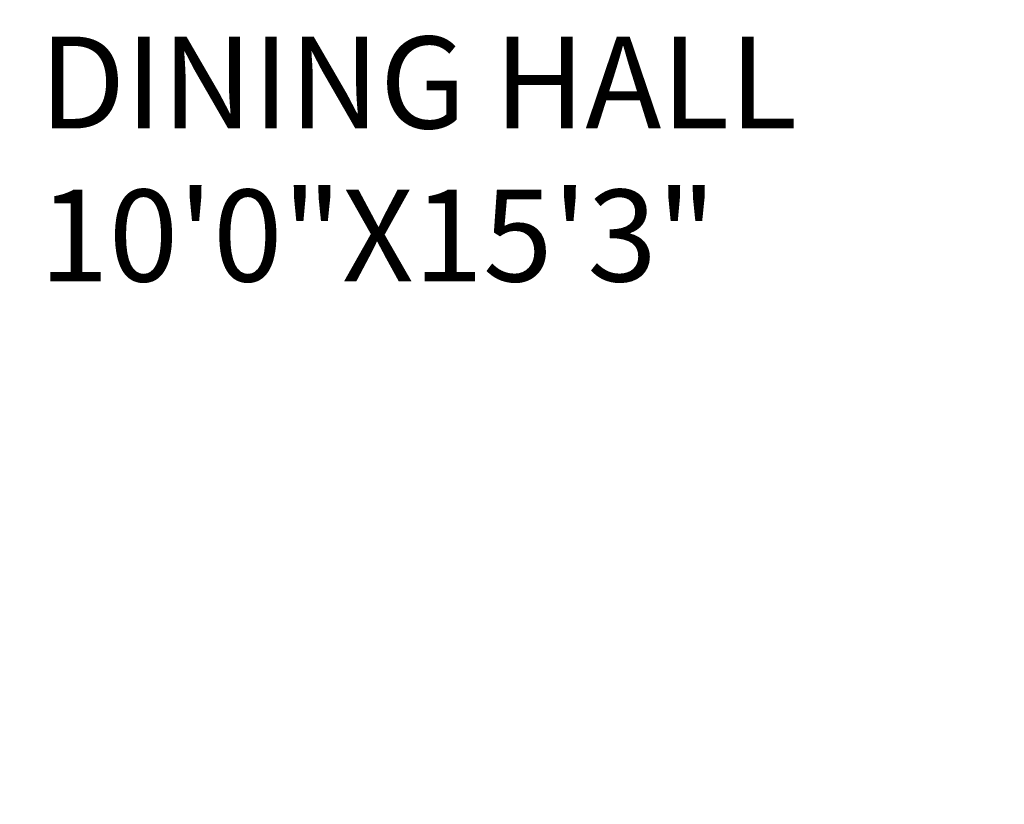
# Model space of a CAD drawing. Units: inches. Extents: x 1088 to 1703, y 668 to 1875.
# Tile 19 of 45: x 1371 to 1436, y 1572 to 1623. Entities that reach past the tile are written whole.
import ezdxf

# ---------------------------------------------------------------- set-up
doc = ezdxf.new("R2010")
doc.units = ezdxf.units.IN
doc.layers.add('A-ANNO-DIMS', color=2, linetype='Continuous', lineweight=18)
doc.layers.add('A-AREA-IDEN', color=7, linetype='Continuous', lineweight=18)
doc.styles.get("Standard").update_dxf_attribs({"font": 'arial.ttf'})
doc.dimstyles.get("Standard").update_dxf_attribs({"dimtxt": 0.18, "dimasz": 0.18, "dimexe": 0.18, "dimexo": 0.0625, "dimgap": 0.09, "dimtad": 0, "dimtih": 1, "dimtoh": 1, "dimdec": 4, "dimzin": 0, "dimdsep": 46, "dimtxsty": 'Standard', "dimcen": 0.09, "dimadec": 0, "dimazin": 0, "dimtfac": 1, "dimtdec": 4, "dimtofl": 0, "dimtmove": 0, "dimatfit": 3, "dimfxl": 1, "dimtolj": 1, "dimtzin": 0, "dimarcsym": 0})

# ---------------------------------------------------------------- blocks, each defined once
blk = doc.blocks.new('*D38')
at = {"layer": 'A-ANNO-DIMS', "color": 0, "lineweight": -2, "transparency": 16777216}
for p, q in [((1317.345, 1736.945), (1317.345, 725.549)), ((1437.345, 1736.945), (1437.345, 725.549)), ((1317.525, 725.729), (1377.065, 725.729)), ((1437.165, 725.729), (1377.625, 725.729))]:
    blk.add_line(p, q, dxfattribs=at)
at = {"layer": 'A-ANNO-DIMS', "color": 0, "transparency": 16777216}
for points in [[(1317.525, 725.759), (1317.525, 725.699), (1317.345, 725.729)], [(1437.165, 725.759), (1437.165, 725.699), (1437.345, 725.729)]]:
    blk.add_solid(points, dxfattribs=at)
at = {"layer": 'Defpoints', "color": 0, "transparency": 16777216}
for p in [(1317.345, 1737.007), (1437.345, 1737.007), (1437.345, 725.729)]:
    blk.add_point(p, dxfattribs=at)
at = {"layer": 'A-ANNO-DIMS', "color": 0, "transparency": 16777216, "insert": (1377.345, 725.729), "char_height": 0.18, "attachment_point": 5}
blk.add_mtext('\\A1;120', dxfattribs=at)

msp = doc.modelspace()

# ---------------------------------------------------------------- texts
at = {"layer": 'A-AREA-IDEN', "insert": (1372.752, 1622.378), "char_height": 6, "attachment_point": 1}
msp.add_mtext_dynamic_manual_height_columns('DINING HALL\\P10\'0"X15\'3"', width=105.30562, gutter_width=12.5, heights=[0], dxfattribs=at)

# ---------------------------------------------------------------- dimensions: what is measured, and where the dimension line sits
at = {"layer": 'A-ANNO-DIMS'}
dim = msp.add_linear_dim(base=(1437.345, 725.729), p1=(1317.345, 1737.007), p2=(1437.345, 1737.007), dimstyle='Standard', override={"dimdec": 0, "dimlfac": 1, "dimrnd": 0, "dimzin": 0, "dimdsep": 46, "dimlunit": 2}, dxfattribs=at)
dim.commit()
dim.dimension.update_dxf_attribs({"geometry": '*D38', "text_midpoint": (1377.345, 725.729)})

doc.saveas('drawing.dxf')
